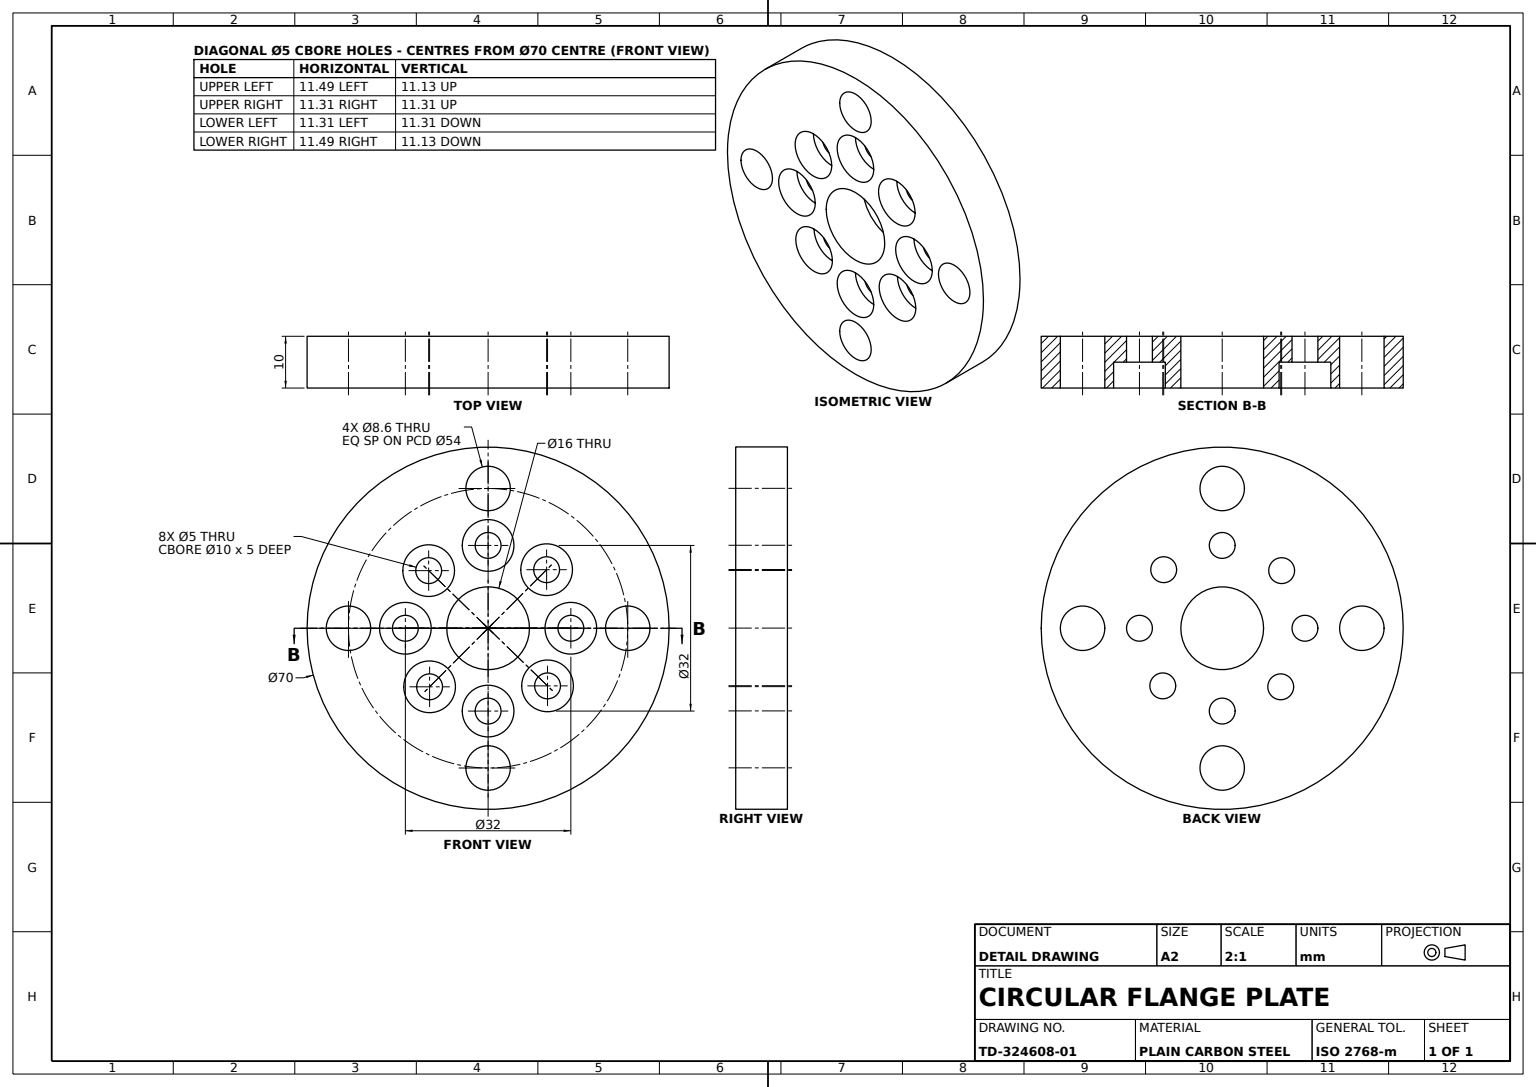
from build123d import *

# Parameters (mm, degrees)
DISC_PROFILE_70_R                  = 35
DISC_70_X_10_DEPTH                 = 10
CENTRE_BORE_PROFILE_16_R           = 8
CENTRE_BORE_16_DEPTH               = 10
OUTER_HOLES_PROFILE_4X_8_6_R       = 4.3
OUTER_HOLES_4X_8_6_DEPTH           = 10
COUNTERBORE_PROFILE_R              = 5
COUNTERBORES_DEPTH_5_DEPTH         = 5
COUNTERBORE_THROUGH_HOLE_PROFILE_R = 2.5
COUNTERBORE_THROUGH_HOLES_DEPTH    = 5


with BuildPart() as part:
    # Disc Profile Ø70 → Disc Ø70 x 10 (new body)
    with BuildSketch(Plane.XY):
        Circle(DISC_PROFILE_70_R)
    extrude(amount=DISC_70_X_10_DEPTH)

    # Centre Bore Profile Ø16 → Centre Bore Ø16 (cut)
    with BuildSketch(Plane.XY.offset(10)):
        Circle(CENTRE_BORE_PROFILE_16_R)
    extrude(amount=-CENTRE_BORE_16_DEPTH, mode=Mode.SUBTRACT)

    # Outer Holes Profile 4xØ8.6 → Outer Holes 4xØ8.6 (cut)
    with BuildSketch(Plane.XY.offset(10)):
        with Locations((0, 27)):
            Circle(OUTER_HOLES_PROFILE_4X_8_6_R)
        with Locations((27, 0)):
            Circle(OUTER_HOLES_PROFILE_4X_8_6_R)
        with Locations((0, -27)):
            Circle(OUTER_HOLES_PROFILE_4X_8_6_R)
        with Locations((-27, 0)):
            Circle(OUTER_HOLES_PROFILE_4X_8_6_R)
    extrude(amount=-OUTER_HOLES_4X_8_6_DEPTH, mode=Mode.SUBTRACT)

    # Counterbore Profile → Counterbores Depth 5 (cut)
    with BuildSketch(Plane.XY.offset(10)):
        with Locations((0, 16)):
            Circle(COUNTERBORE_PROFILE_R)
        with Locations((16, 0)):
            Circle(COUNTERBORE_PROFILE_R)
        with Locations((0, -16)):
            Circle(COUNTERBORE_PROFILE_R)
        with Locations((-16, 0)):
            Circle(COUNTERBORE_PROFILE_R)
        with Locations((11.492535714, -11.132008932)):
            Circle(COUNTERBORE_PROFILE_R)
        with Locations((11.313708499, 11.313708499)):
            Circle(COUNTERBORE_PROFILE_R)
        with Locations((-11.492535714, 11.132008932)):
            Circle(COUNTERBORE_PROFILE_R)
        with Locations((-11.313708499, -11.313708499)):
            Circle(COUNTERBORE_PROFILE_R)
    extrude(amount=-COUNTERBORES_DEPTH_5_DEPTH, mode=Mode.SUBTRACT)

    # Counterbore Through Hole Profile → Counterbore Through Holes (cut)
    with BuildSketch(Plane.XY.offset(5)):
        with Locations((0, 16)):
            Circle(COUNTERBORE_THROUGH_HOLE_PROFILE_R)
        with Locations((11.313708499, 11.313708499)):
            Circle(COUNTERBORE_THROUGH_HOLE_PROFILE_R)
        with Locations((16, 0)):
            Circle(COUNTERBORE_THROUGH_HOLE_PROFILE_R)
        with Locations((11.492535714, -11.132008932)):
            Circle(COUNTERBORE_THROUGH_HOLE_PROFILE_R)
        with Locations((0, -16)):
            Circle(COUNTERBORE_THROUGH_HOLE_PROFILE_R)
        with Locations((-11.313708499, -11.313708499)):
            Circle(COUNTERBORE_THROUGH_HOLE_PROFILE_R)
        with Locations((-16, 0)):
            Circle(COUNTERBORE_THROUGH_HOLE_PROFILE_R)
        with Locations((-11.492535714, 11.132008932)):
            Circle(COUNTERBORE_THROUGH_HOLE_PROFILE_R)
    extrude(amount=-COUNTERBORE_THROUGH_HOLES_DEPTH, mode=Mode.SUBTRACT)


solid = part.part
